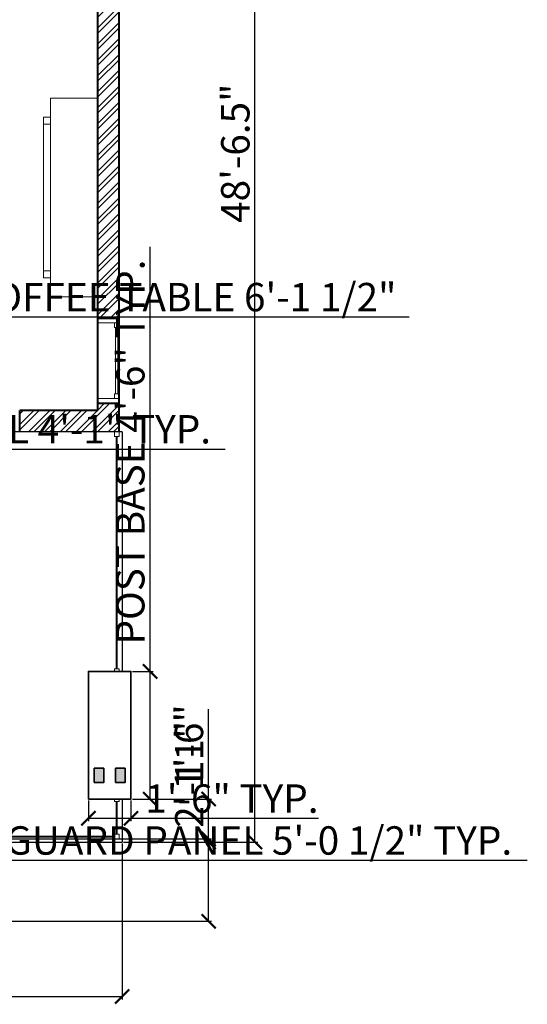
# Model space of a CAD drawing. Units: inches. Extents: x 982 to 1904, y 735 to 1463.
# Tile 6 of 7: x 1689 to 1904, y 744 to 1160. Entities that reach past the tile are written whole.
import ezdxf

# ---------------------------------------------------------------- set-up
doc = ezdxf.new("R2010")
doc.units = ezdxf.units.IN
for name, color, linetype, lineweight in [('A-COLS', 7, 'Continuous', 35), ('A-FLOR', 7, 'Continuous', 25), ('A-FLOR-RAIL', 7, 'Continuous', 18), ('Dimensions', 9, 'Continuous', 18), ('Furniture', 31, 'Continuous', 18), ('Wall Hatch', 23, 'Continuous', 13), ('Walls', 151, 'Continuous', 40), ('Windows', 111, 'Continuous', 18)]:
    doc.layers.add(name, color=color, linetype=linetype, lineweight=lineweight)
doc.layers.add('A-COLS-PATT', color=251, linetype='Continuous', lineweight=13, true_color=0x636466)
doc.styles.get("Standard").update_dxf_attribs({"font": 'arial.ttf'})
doc.dimstyles.new('ISO-25', dxfattribs={"dimtxt": 12, "dimasz": 6, "dimexe": 1.25, "dimexo": 0.625, "dimtad": 1, "dimlunit": 3, "dimtxsty": 'Standard', "dimblk": 'ARCHTICK', "dimcen": 2.5, "dimadec": 0, "dimazin": 0, "dimtfac": 1, "dimtmove": 0, "dimatfit": 3, "dimfxl": 1, "dimarcsym": 0})

# ---------------------------------------------------------------- blocks, each defined once
blk = doc.blocks.new('_ArchTick')
at = {"color": 0, "linetype": 'ByBlock', "const_width": 0.15}
blk.add_lwpolyline([(-0.5, -0.5), (0.5, 0.5)], dxfattribs=at)
blk = doc.blocks.new('*D22')
at = {"layer": 'Defpoints', "color": 0, "transparency": 16777216}
for p in [(1156.5, 893.99), (1732.75, 812.49), (1732.75, 747.2)]:
    blk.add_point(p, dxfattribs=at)
at = {"layer": 'Dimensions', "color": 0, "lineweight": -2, "transparency": 16777216}
for p, q in [((1156.5, 893.37), (1156.5, 745.95)), ((1732.75, 811.87), (1732.75, 745.95)), ((1156.5, 747.2), (1732.75, 747.2))]:
    blk.add_line(p, q, dxfattribs=at)
at = {"layer": 'Dimensions', "color": 0, "lineweight": -2, "transparency": 16777216, "xscale": 6, "yscale": 6, "zscale": 6, "rotation": 180}
blk.add_blockref('_ArchTick', (1156.5, 747.2), dxfattribs=at)
at = {"layer": 'Dimensions', "color": 0, "lineweight": -2, "transparency": 16777216, "xscale": 6, "yscale": 6, "zscale": 6}
blk.add_blockref('_ArchTick', (1732.75, 747.2), dxfattribs=at)
at = {"layer": 'Dimensions', "color": 0, "transparency": 16777216, "insert": (1444.62, 753.95), "char_height": 12, "attachment_point": 5}
blk.add_mtext('48\'-0.25"', dxfattribs=at)
blk = doc.blocks.new('*D23')
at = {"layer": 'Defpoints', "color": 0, "transparency": 16777216}
for p in [(1731.5, 1394.99), (1788.92, 1394.99), (1732.75, 812.49)]:
    blk.add_point(p, dxfattribs=at)
at = {"layer": 'Dimensions', "color": 0, "lineweight": -2, "transparency": 16777216}
for p, q in [((1732.12, 1394.99), (1790.17, 1394.99)), ((1788.92, 812.49), (1788.92, 1394.99)), ((1733.37, 812.49), (1790.17, 812.49))]:
    blk.add_line(p, q, dxfattribs=at)
at = {"layer": 'Dimensions', "color": 0, "lineweight": -2, "transparency": 16777216, "xscale": 6, "yscale": 6, "zscale": 6}
for p, rotation in [((1788.92, 1394.99), 90), ((1788.92, 812.49), 270)]:
    blk.add_blockref('_ArchTick', p, dxfattribs=dict(at, rotation=rotation))
at = {"layer": 'Dimensions', "color": 0, "transparency": 16777216, "insert": (1782.16, 1103.74), "char_height": 12, "attachment_point": 5, "rotation": 90}
blk.add_mtext('48\'-6.5"', dxfattribs=at)
blk = doc.blocks.new('POST-BASE-18x54')
for points in [[(0, 0), (18, 0), (18, 54), (0, 54)], [(2.5, 7), (6.5, 7), (6.5, 13), (2.5, 13)], [(11.5, 7), (15.5, 7), (15.5, 13), (11.5, 13)]]:
    blk.add_lwpolyline(points, close=True)
blk = doc.blocks.new('GUARD-PANEL-60_5')
for p, q in [((0, 1.16), (58.5, 1.16)), ((0, 0.66), (58.5, 0.66))]:
    blk.add_line(p, q)
blk.add_lwpolyline([(58.5, 2), (60.5, 2), (60.5, 0), (58.5, 0)], close=True)
blk = doc.blocks.new('*D28')
at = {"layer": 'Defpoints', "color": 0, "transparency": 16777216}
for p in [(1610.5, 813.83), (1671, 813.83), (1671, 804.76)]:
    blk.add_point(p, dxfattribs=at)
at = {"layer": 'Dimensions', "color": 0, "lineweight": -2, "transparency": 16777216}
for p, q in [((1610.5, 813.21), (1610.5, 803.51)), ((1671, 813.21), (1671, 803.51)), ((1610.5, 804.76), (1671, 804.76)), ((1671, 804.76), (1903.99, 804.76))]:
    blk.add_line(p, q, dxfattribs=at)
at = {"layer": 'Dimensions', "color": 0, "lineweight": -2, "transparency": 16777216, "xscale": 6, "yscale": 6, "zscale": 6, "rotation": 180}
blk.add_blockref('_ArchTick', (1610.5, 804.76), dxfattribs=at)
at = {"layer": 'Dimensions', "color": 0, "lineweight": -2, "transparency": 16777216, "xscale": 6, "yscale": 6, "zscale": 6}
blk.add_blockref('_ArchTick', (1671, 804.76), dxfattribs=at)
at = {"layer": 'Dimensions', "color": 0, "transparency": 16777216, "insert": (1790.49, 811.59), "char_height": 12, "attachment_point": 5}
blk.add_mtext('GUARD PANEL 5\'-0 1/2" TYP.', dxfattribs=at)
blk = doc.blocks.new('*D29')
at = {"layer": 'Defpoints', "color": 0, "transparency": 16777216}
for p in [(1671, 815.83), (1671, 813.83), (1680.07, 815.83)]:
    blk.add_point(p, dxfattribs=at)
at = {"layer": 'Dimensions', "color": 0, "lineweight": -2, "transparency": 16777216}
for p, q in [((1680.07, 815.83), (1680.07, 896.23)), ((1671.62, 815.83), (1681.32, 815.83)), ((1671.62, 813.83), (1681.32, 813.83)), ((1680.07, 813.83), (1680.07, 815.83))]:
    blk.add_line(p, q, dxfattribs=at)
at = {"layer": 'Dimensions', "color": 0, "lineweight": -2, "transparency": 16777216, "xscale": 6, "yscale": 6, "zscale": 6}
for p, rotation in [((1680.07, 815.83), 90), ((1680.07, 813.83), 270)]:
    blk.add_blockref('_ArchTick', p, dxfattribs=dict(at, rotation=rotation))
at = {"layer": 'Dimensions', "color": 0, "transparency": 16777216, "insert": (1673.32, 859.03), "char_height": 12, "attachment_point": 5, "rotation": 90}
blk.add_mtext('0\'-2" TYP.', dxfattribs=at)
blk = doc.blocks.new('*D32')
at = {"layer": 'Defpoints', "color": 0, "transparency": 16777216}
for p in [(1736.52, 884.66), (1744.62, 884.66), (1736.52, 830.66)]:
    blk.add_point(p, dxfattribs=at)
at = {"layer": 'Dimensions', "color": 0, "lineweight": -2, "transparency": 16777216}
for p, q in [((1744.62, 884.66), (1744.62, 1064.14)), ((1737.14, 884.66), (1745.87, 884.66)), ((1744.62, 830.66), (1744.62, 884.66)), ((1737.14, 830.66), (1745.87, 830.66))]:
    blk.add_line(p, q, dxfattribs=at)
at = {"layer": 'Dimensions', "color": 0, "lineweight": -2, "transparency": 16777216, "xscale": 6, "yscale": 6, "zscale": 6}
for p, rotation in [((1744.62, 884.66), 90), ((1744.62, 830.66), 270)]:
    blk.add_blockref('_ArchTick', p, dxfattribs=dict(at, rotation=rotation))
at = {"layer": 'Dimensions', "color": 0, "transparency": 16777216, "insert": (1737.79, 977.4), "char_height": 12, "attachment_point": 5, "rotation": 90}
blk.add_mtext('POST BASE 4\'-6" TYP.', dxfattribs=at)
blk = doc.blocks.new('*D33')
at = {"layer": 'Defpoints', "color": 0, "transparency": 16777216}
for p in [(1718.52, 830.66), (1736.52, 830.66), (1736.52, 822.56)]:
    blk.add_point(p, dxfattribs=at)
at = {"layer": 'Dimensions', "color": 0, "lineweight": -2, "transparency": 16777216}
for p, q in [((1718.52, 830.03), (1718.52, 821.31)), ((1736.52, 830.03), (1736.52, 821.31)), ((1718.52, 822.56), (1736.52, 822.56)), ((1736.52, 822.56), (1815.79, 822.56))]:
    blk.add_line(p, q, dxfattribs=at)
at = {"layer": 'Dimensions', "color": 0, "lineweight": -2, "transparency": 16777216, "xscale": 6, "yscale": 6, "zscale": 6, "rotation": 180}
blk.add_blockref('_ArchTick', (1718.52, 822.56), dxfattribs=at)
at = {"layer": 'Dimensions', "color": 0, "lineweight": -2, "transparency": 16777216, "xscale": 6, "yscale": 6, "zscale": 6}
blk.add_blockref('_ArchTick', (1736.52, 822.56), dxfattribs=at)
at = {"layer": 'Dimensions', "color": 0, "transparency": 16777216, "insert": (1779.15, 829.31), "char_height": 12, "attachment_point": 5}
blk.add_mtext('1\'-6" TYP.', dxfattribs=at)
blk = doc.blocks.new('*D38')
at = {"layer": 'Defpoints', "color": 0, "transparency": 16777216}
for p in [(1515.5, 985.99), (1564.55, 985.99), (1564.55, 978.63)]:
    blk.add_point(p, dxfattribs=at)
at = {"layer": 'Dimensions', "color": 0, "lineweight": -2, "transparency": 16777216}
for p, q in [((1515.5, 985.37), (1515.5, 977.38)), ((1564.55, 985.37), (1564.55, 977.38)), ((1515.5, 978.63), (1564.55, 978.63)), ((1564.55, 978.63), (1776.25, 978.63))]:
    blk.add_line(p, q, dxfattribs=at)
at = {"layer": 'Dimensions', "color": 0, "lineweight": -2, "transparency": 16777216, "xscale": 6, "yscale": 6, "zscale": 6, "rotation": 180}
blk.add_blockref('_ArchTick', (1515.5, 978.63), dxfattribs=at)
at = {"layer": 'Dimensions', "color": 0, "lineweight": -2, "transparency": 16777216, "xscale": 6, "yscale": 6, "zscale": 6}
blk.add_blockref('_ArchTick', (1564.55, 978.63), dxfattribs=at)
at = {"layer": 'Dimensions', "color": 0, "transparency": 16777216, "insert": (1673.4, 985.46), "char_height": 12, "attachment_point": 5}
blk.add_mtext('SLIDING PANEL 4\'-1" TYP.', dxfattribs=at)
blk = doc.blocks.new('*D46')
at = {"layer": 'Defpoints', "color": 0, "transparency": 16777216}
for p in [(1583.35, 1045.5), (1656.61, 1045.5), (1656.61, 1034.51)]:
    blk.add_point(p, dxfattribs=at)
at = {"layer": 'Dimensions', "color": 0, "lineweight": -2, "transparency": 16777216}
for p, q in [((1583.35, 1044.87), (1583.35, 1033.26)), ((1656.61, 1044.87), (1656.61, 1033.26)), ((1583.35, 1034.51), (1656.61, 1034.51)), ((1656.61, 1034.51), (1854, 1034.51))]:
    blk.add_line(p, q, dxfattribs=at)
at = {"layer": 'Dimensions', "color": 0, "lineweight": -2, "transparency": 16777216, "xscale": 6, "yscale": 6, "zscale": 6, "rotation": 180}
blk.add_blockref('_ArchTick', (1583.35, 1034.51), dxfattribs=at)
at = {"layer": 'Dimensions', "color": 0, "lineweight": -2, "transparency": 16777216, "xscale": 6, "yscale": 6, "zscale": 6}
blk.add_blockref('_ArchTick', (1656.61, 1034.51), dxfattribs=at)
at = {"layer": 'Dimensions', "color": 0, "transparency": 16777216, "insert": (1758.31, 1041.34), "char_height": 12, "attachment_point": 5}
blk.add_mtext('COFFEE TABLE 6\'-1 1/2"', dxfattribs=at)
blk = doc.blocks.new('*D54')
at = {"layer": 'Defpoints', "color": 0, "transparency": 16777216}
for p in [(1489.5, 813.83), (1769.32, 813.83), (1494.68, 778.99)]:
    blk.add_point(p, dxfattribs=at)
at = {"layer": 'Dimensions', "color": 0, "lineweight": -2, "transparency": 16777216}
for p, q in [((1769.32, 813.83), (1769.32, 862.51)), ((1490.12, 813.83), (1770.57, 813.83)), ((1769.32, 778.99), (1769.32, 813.83)), ((1495.3, 778.99), (1770.57, 778.99))]:
    blk.add_line(p, q, dxfattribs=at)
at = {"layer": 'Dimensions', "color": 0, "lineweight": -2, "transparency": 16777216, "xscale": 6, "yscale": 6, "zscale": 6}
for p, rotation in [((1769.32, 813.83), 90), ((1769.32, 778.99), 270)]:
    blk.add_blockref('_ArchTick', p, dxfattribs=dict(at, rotation=rotation))
at = {"layer": 'Dimensions', "color": 0, "transparency": 16777216, "insert": (1762.67, 841.17), "char_height": 12, "attachment_point": 5, "rotation": 90}
blk.add_mtext('2\'-11"', dxfattribs=at)
blk = doc.blocks.new('*D72')
at = {"layer": 'Defpoints', "color": 0, "transparency": 16777216}
for p in [(1736.52, 830.66), (1769.32, 830.66), (1732.75, 812.49)]:
    blk.add_point(p, dxfattribs=at)
at = {"layer": 'Dimensions', "color": 0, "lineweight": -2, "transparency": 16777216}
for p, q in [((1769.32, 830.66), (1769.32, 868.68)), ((1737.14, 830.66), (1770.57, 830.66)), ((1769.32, 812.49), (1769.32, 830.66)), ((1733.37, 812.49), (1770.57, 812.49))]:
    blk.add_line(p, q, dxfattribs=at)
at = {"layer": 'Dimensions', "color": 0, "lineweight": -2, "transparency": 16777216, "xscale": 6, "yscale": 6, "zscale": 6}
for p, rotation in [((1769.32, 830.66), 90), ((1769.32, 812.49), 270)]:
    blk.add_blockref('_ArchTick', p, dxfattribs=dict(at, rotation=rotation))
at = {"layer": 'Dimensions', "color": 0, "transparency": 16777216, "insert": (1762.57, 852.67), "char_height": 12, "attachment_point": 5, "rotation": 90}
blk.add_mtext('1\'-6"', dxfattribs=at)

msp = doc.modelspace()

# ---------------------------------------------------------------- hatches: boundary and pattern name
at = {"layer": 'A-COLS-PATT'}
h = msp.add_hatch(color=256, dxfattribs=at)
h.dxf.hatch_style = 1
h.paths.add_polyline_path([(1731.496, 1394.991), (1722.496, 1394.991), (1722.496, 1385.991), (1731.496, 1385.991)])
h.paths.add_polyline_path([(1725.019, 843.656), (1721.019, 843.656), (1721.019, 837.656), (1725.019, 837.656)])
h.paths.add_polyline_path([(1734.019, 843.656), (1730.019, 843.656), (1730.019, 837.656), (1734.019, 837.656)])
h.paths.add_polyline_path([(1483.18, 791.991), (1479.18, 791.991), (1479.18, 785.991), (1483.18, 785.991)])
h.paths.add_polyline_path([(1492.18, 791.991), (1488.18, 791.991), (1488.18, 785.991), (1492.18, 785.991)])
h.paths.add_polyline_path([(1364.813, 791.991), (1360.813, 791.991), (1360.813, 785.991), (1364.813, 785.991)])
h.paths.add_polyline_path([(1373.813, 791.991), (1369.813, 791.991), (1369.813, 785.991), (1373.813, 785.991)])
at = {"layer": 'Wall Hatch'}
h = msp.add_hatch(dxfattribs=at)
h.set_pattern_fill('ANSI32', color=256, scale=0.5)
h.paths.add_polyline_path([(1165.496, 1065.991), (1271.496, 1065.991), (1271.496, 1071.991), (1218.496, 1071.991), (1218.496, 1238.491), (1262.496, 1238.491), (1262.496, 1244.491), (1218.496, 1244.491), (1218.496, 1330.491), (1298.496, 1330.491), (1298.496, 1244.491), (1292.496, 1244.491), (1292.496, 1238.491), (1298.496, 1238.491), (1298.496, 1221.991), (1304.496, 1221.991), (1304.496, 1224.991), (1374.496, 1224.991), (1374.496, 1230.991), (1304.496, 1230.991), (1304.496, 1251.991), (1310.496, 1251.991), (1310.496, 1257.991), (1304.496, 1257.991), (1304.496, 1385.991), (1328.496, 1385.991), (1328.496, 1394.991), (1295.496, 1394.991), (1295.496, 1339.491), (1209.496, 1339.491), (1209.496, 1071.991), (1156.496, 1071.991), (1156.496, 893.991), (1171.496, 893.991), (1171.496, 902.991), (1165.496, 902.991)])
h.paths.add_polyline_path([(1273.996, 877.991), (1267.996, 877.991), (1267.996, 902.991), (1252.996, 902.991), (1252.996, 893.991), (1258.996, 893.991), (1258.996, 868.991), (1273.996, 868.991)])
h.paths.add_polyline_path([(1370.496, 1052.991), (1361.496, 1052.991), (1361.496, 1046.991), (1355.496, 1046.991), (1355.496, 1040.991), (1361.496, 1040.991), (1361.496, 877.991), (1355.496, 877.991), (1355.496, 868.991), (1361.496, 868.991), (1361.496, 832.991), (1376.313, 832.991), (1491.496, 832.991), (1491.496, 985.991), (1515.496, 985.991), (1515.496, 994.991), (1482.496, 994.991), (1482.496, 841.991), (1370.496, 841.991)])
h.paths.add_polyline_path([(1319.496, 1088.991), (1325.496, 1088.991), (1325.496, 1094.991), (1319.496, 1094.991), (1319.496, 1112.491), (1361.496, 1112.491), (1361.496, 1094.991), (1355.496, 1094.991), (1355.496, 1088.991), (1361.496, 1088.991), (1361.496, 1082.991), (1370.496, 1082.991), (1370.496, 1180.991), (1503.496, 1180.991), (1503.496, 1231.991), (1497.496, 1231.991), (1497.496, 1215.991), (1491.496, 1215.991), (1491.496, 1209.991), (1497.496, 1209.991), (1497.496, 1189.991), (1448.496, 1189.991), (1448.496, 1209.991), (1454.496, 1209.991), (1454.496, 1215.991), (1448.496, 1215.991), (1448.496, 1221.991), (1442.496, 1221.991), (1442.496, 1189.991), (1380.496, 1189.991), (1380.496, 1251.991), (1442.496, 1251.991), (1442.496, 1245.991), (1448.496, 1245.991), (1448.496, 1263.991), (1442.496, 1263.991), (1442.496, 1257.991), (1368.496, 1257.991), (1368.496, 1251.991), (1374.496, 1251.991), (1374.496, 1189.991), (1304.496, 1189.991), (1304.496, 1192.991), (1295.496, 1192.991), (1295.496, 1183.991), (1361.496, 1183.991), (1361.496, 1118.491), (1313.496, 1118.491), (1313.496, 1071.991), (1301.496, 1071.991), (1301.496, 1065.991), (1313.496, 1065.991), (1313.496, 1040.991), (1325.496, 1040.991), (1325.496, 1046.991), (1319.496, 1046.991)])
h.paths.add_polyline_path([(1565.496, 1394.991), (1418.496, 1394.991), (1418.496, 1385.991), (1442.496, 1385.991), (1442.496, 1293.991), (1448.496, 1293.991), (1448.496, 1299.991), (1454.496, 1299.991), (1454.496, 1305.991), (1448.496, 1305.991), (1448.496, 1385.991), (1556.496, 1385.991), (1556.496, 1307.991), (1497.496, 1307.991), (1497.496, 1305.991), (1491.496, 1305.991), (1491.496, 1299.991), (1497.496, 1299.991), (1497.496, 1268.991), (1503.496, 1268.991), (1503.496, 1298.991), (1656.496, 1298.991), (1656.496, 1307.991), (1565.496, 1307.991)])
h.paths.add_polyline_path([(1731.496, 1307.991), (1698.496, 1307.991), (1698.496, 1298.991), (1722.496, 1298.991), (1722.496, 1033.991), (1731.496, 1033.991)])
h.paths.add_polyline_path([(1731.496, 997.991), (1722.496, 997.991), (1722.496, 994.991), (1689.496, 994.991), (1689.496, 985.991), (1731.496, 985.991)])

# ---------------------------------------------------------------- linework, layer by layer
at = {"layer": 'A-FLOR'}
for p, q in [((1732.746, 985.991), (1491.496, 985.991)), ((1732.746, 985.991), (1732.746, 884.656)), ((1732.746, 830.656), (1732.746, 812.491)), ((1494.68, 812.491), (1732.746, 812.491))]:
    msp.add_line(p, q, dxfattribs=at)
at = {"layer": 'A-FLOR-RAIL'}
for p, q in [((1730.246, 983.991), (1730.246, 885.656)), ((1730.746, 983.991), (1730.746, 885.656)), ((1730.246, 829.656), (1730.246, 815.833)), ((1730.746, 829.656), (1730.746, 815.833)), ((1731.496, 814.991), (1731.496, 815.833))]:
    msp.add_line(p, q, dxfattribs=at)
msp.add_lwpolyline([(1729.496, 985.991), (1731.496, 985.991), (1731.496, 983.991), (1729.496, 983.991)], close=True, dxfattribs=at)
for points in [[(1729.496, 884.656), (1729.496, 885.656), (1731.496, 885.656), (1731.496, 884.656)], [(1731.496, 830.656), (1731.496, 829.656), (1729.496, 829.656), (1729.496, 830.656)]]:
    msp.add_lwpolyline(points, dxfattribs=at)
at = {"layer": 'Furniture'}
for p, q in [((1702.496, 1042.991), (1702.496, 1126.991)), ((1722.496, 1126.991), (1702.496, 1126.991)), ((1699.496, 1050.991), (1699.496, 1118.991)), ((1702.496, 1118.991), (1699.496, 1118.991)), ((1702.496, 1115.991), (1699.496, 1115.991)), ((1702.496, 1053.991), (1699.496, 1053.991)), ((1702.496, 1050.991), (1699.496, 1050.991)), ((1722.496, 1042.991), (1702.496, 1042.991))]:
    msp.add_line(p, q, dxfattribs=at)
at = {"layer": 'Walls'}
for p, q in [((1731.496, 985.991), (1731.496, 1307.991)), ((1722.496, 994.991), (1722.496, 1298.991)), ((1722.496, 1033.991), (1731.496, 1033.991)), ((1722.496, 997.991), (1731.496, 997.991)), ((1722.496, 994.991), (1689.496, 994.991)), ((1689.496, 985.991), (1689.496, 994.991))]:
    msp.add_line(p, q, dxfattribs=at)
at = {"layer": 'Windows'}
for p, q in [((1722.496, 1031.991), (1731.496, 1031.991)), ((1729.996, 1001.991), (1729.996, 1029.991)), ((1730.996, 1001.991), (1730.996, 1029.991)), ((1722.496, 999.991), (1731.496, 999.991))]:
    msp.add_line(p, q, dxfattribs=at)
for points in [[(1729.496, 1029.991), (1731.496, 1029.991), (1731.496, 1031.991), (1729.496, 1031.991)], [(1729.496, 1001.991), (1731.496, 1001.991), (1731.496, 999.991), (1729.496, 999.991)]]:
    msp.add_lwpolyline(points, close=True, dxfattribs=at)

# ---------------------------------------------------------------- block references
at = {"layer": 'A-COLS'}
msp.add_blockref('POST-BASE-18x54', (1718.519, 830.656), dxfattribs=at)
at = {"layer": 'A-FLOR-RAIL'}
msp.add_blockref('GUARD-PANEL-60_5', (1670.996, 813.833), dxfattribs=at)

# ---------------------------------------------------------------- dimensions: what is measured, and where the dimension line sits
at = {"layer": 'Dimensions'}
for base, p1, p2, override, picture, middle in [((1788.915, 1394.991), (1732.746, 812.491), (1731.496, 1394.991), {"dimclrd": 0, "dimclre": 0, "dimclrt": 0}, '*D23', (1782.164, 1103.741)), ((1769.319, 830.656), (1732.746, 812.491), (1736.519, 830.656), {"dimdec": 1, "dimlfac": 1, "dimrnd": 0, "dimzin": 1, "dimdsep": 46, "dimlunit": 4, "dimfrac": 2}, '*D72', (1762.567, 852.666)), ((1769.319, 813.833), (1494.68, 778.991), (1489.496, 813.833), {"dimdec": 1, "dimlfac": 1, "dimrnd": 0, "dimzin": 1, "dimdsep": 46, "dimlunit": 4, "dimfrac": 2}, '*D54', (1762.669, 841.172))]:
    dim = msp.add_linear_dim(base=base, p1=p1, p2=p2, angle=90, dimstyle='ISO-25', override=override, dxfattribs=at)
    dim.commit()
    dim.dimension.update_dxf_attribs({"geometry": picture, "text_midpoint": middle})
for base, p1, p2, text, picture, middle in [((1656.614, 1034.508), (1583.351, 1045.497), (1656.614, 1045.497), 'COFFEE TABLE <>', '*D46', (1758.306, 1041.342)), ((1564.5456, 978.6336), (1515.4964, 985.991), (1564.5456, 985.991), 'SLIDING PANEL <> TYP.', '*D38', (1673.3957, 985.4632)), ((1670.996, 804.758), (1610.496, 813.833), (1670.996, 813.833), 'GUARD PANEL <> TYP.', '*D28', (1790.492, 811.588)), ((1736.519, 822.556), (1718.519, 830.656), (1736.519, 830.656), '<> TYP.', '*D33', (1779.152, 829.308))]:
    dim = msp.add_linear_dim(base=base, p1=p1, p2=p2, text=text, dimstyle='ISO-25', override={"dimdec": 1, "dimlfac": 1, "dimrnd": 0, "dimzin": 1, "dimdsep": 46, "dimlunit": 4, "dimfrac": 2}, dxfattribs=at)
    dim.commit()
    dim.dimension.update_dxf_attribs({"geometry": picture, "text_midpoint": middle})
for base, p1, p2, text, picture, middle in [((1744.619, 884.656), (1736.519, 830.656), (1736.519, 884.656), 'POST BASE <> TYP.', '*D32', (1737.785, 977.397)), ((1680.071, 815.833), (1670.996, 813.833), (1670.996, 815.833), '<> TYP.', '*D29', (1673.32, 859.031))]:
    dim = msp.add_linear_dim(base=base, p1=p1, p2=p2, angle=90, text=text, dimstyle='ISO-25', override={"dimdec": 1, "dimlfac": 1, "dimrnd": 0, "dimzin": 1, "dimdsep": 46, "dimlunit": 4, "dimfrac": 2}, dxfattribs=at)
    dim.commit()
    dim.dimension.update_dxf_attribs({"geometry": picture, "text_midpoint": middle})
dim = msp.add_linear_dim(base=(1732.746, 747.196), p1=(1156.496, 893.991), p2=(1732.746, 812.491), dimstyle='ISO-25', override={"dimclrd": 0, "dimclre": 0, "dimclrt": 0}, dxfattribs=at)
dim.commit()
dim.dimension.update_dxf_attribs({"geometry": '*D22', "text_midpoint": (1444.621, 753.948)})

doc.saveas('drawing.dxf')
